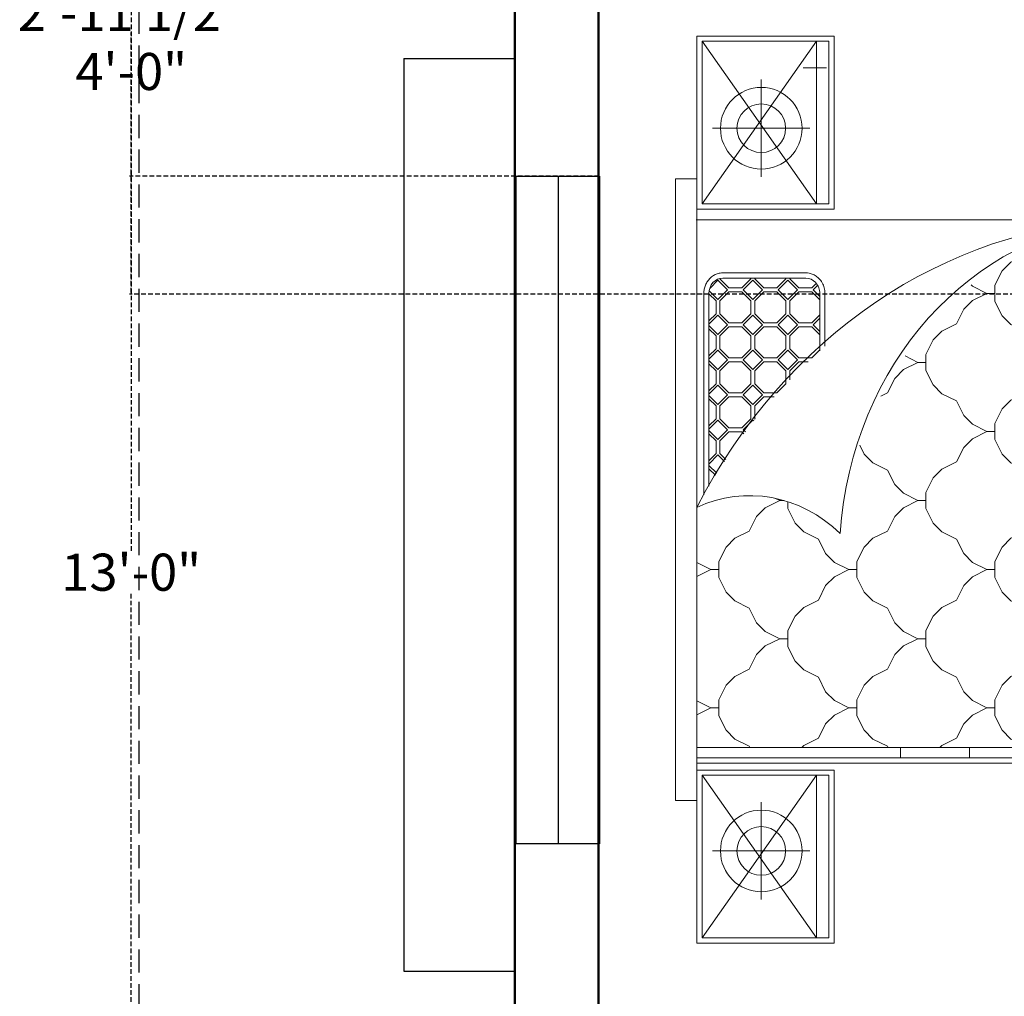
# Model space of a CAD drawing. Units: inches. Extents: x 513 to 1142, y 396 to 927.
# Tile 6 of 31: x 522 to 628, y 746 to 852. Entities that reach past the tile are written whole.
import ezdxf

# ---------------------------------------------------------------- set-up
doc = ezdxf.new("R2010")
doc.units = ezdxf.units.IN
doc.header["$MEASUREMENT"] = 0
doc.linetypes.add('DASHED', pattern=[0.75, 0.5, -0.25])
for name, color, linetype, lineweight in [('A-ANNO-DIMS', 2, 'DASHED', 18), ('A-WALL', 7, 'Continuous', 50), ('furniture', 92, 'Continuous', 18), ('windows', 172, 'Continuous', 25)]:
    doc.layers.add(name, color=color, linetype=linetype, lineweight=lineweight)
doc.styles.get("Standard").update_dxf_attribs({"font": 'arial.ttf'})
doc.dimstyles.get("Standard").update_dxf_attribs({"dimtxt": 4, "dimasz": 0.18, "dimexe": 0.18, "dimexo": 0.0625, "dimgap": 0.09, "dimtad": 0, "dimtih": 1, "dimtoh": 1, "dimdec": 0, "dimrnd": 6, "dimzin": 0, "dimdsep": 46, "dimlunit": 3, "dimtxsty": 'Standard', "dimcen": 0.09, "dimadec": 0, "dimazin": 0, "dimtfac": 1, "dimtdec": 0, "dimtofl": 0, "dimtmove": 0, "dimatfit": 3, "dimfxl": 1, "dimtolj": 1, "dimtzin": 0, "dimarcsym": 0})

# ---------------------------------------------------------------- blocks, each defined once
blk = doc.blocks.new('A$C029D5C69')
for p, q in [((0.4164, 2.0693), (0.4164, 2.0066)), ((2.2315, 2.0693), (0.4164, 2.0693)), ((2.2315, 2.0066), (2.2315, 2.0693)), ((0, 1.606), (0, 2.0066)), ((0, 2.0066), (0.505, 2.0066)), ((0.0151, 1.6211), (0.0151, 1.9915)), ((0.0151, 1.9915), (0.4899, 1.9915)), ((0.4164, 2.0066), (2.2315, 2.0066)), ((0.4899, 1.9915), (0.4899, 1.6211)), ((0.505, 2.0066), (0.505, 1.606)), ((0.5252, 0.0351), (0.5252, 2.0066)), ((0.5403, 0.0502), (0.5403, 2.0066)), ((0.5706, 0.0805), (0.5706, 2.0066)), ((0.6869, 1.966), (0.6666, 2.0066)), ((0.7072, 2.0066), (0.6869, 1.966)), ((1.0902, 1.966), (1.0699, 2.0066)), ((1.1106, 2.0066), (1.0902, 1.966)), ((1.8954, 1.9865), (1.3081, 1.9865)), ((2.1114, 2.0087), (2.1114, 0.0351)), ((2.6479, 2.0066), (2.1429, 2.0066)), ((2.1429, 2.0066), (2.1429, 1.606)), ((2.6328, 1.9915), (2.158, 1.9915)), ((2.158, 1.9915), (2.158, 1.6211)), ((2.6328, 1.6211), (2.6328, 1.9915)), ((2.6479, 1.606), (2.6479, 2.0066)), ((0.2689, 1.9609), (0.2689, 1.6764)), ((0.6869, 1.9425), (0.6869, 1.966)), ((0.6869, 1.9425), (0.6869, 1.966)), ((1.0902, 1.9425), (1.0902, 1.966)), ((1.0902, 1.9425), (1.0902, 1.966)), ((1.8954, 1.9713), (1.3339, 1.9713)), ((1.3849, 1.9713), (1.3656, 1.952)), ((1.3945, 1.9713), (1.3714, 1.9483)), ((1.4249, 1.945), (1.3986, 1.9713)), ((1.4288, 1.9507), (1.4081, 1.9713)), ((1.487, 1.9713), (1.4664, 1.9507)), ((1.4966, 1.9713), (1.4703, 1.945)), ((1.527, 1.945), (1.5007, 1.9713)), ((1.5309, 1.9507), (1.5102, 1.9713)), ((1.5891, 1.9713), (1.5685, 1.9507)), ((1.5987, 1.9713), (1.5724, 1.945)), ((1.6291, 1.945), (1.6028, 1.9713)), ((1.633, 1.9507), (1.6123, 1.9713)), ((1.6912, 1.9713), (1.6706, 1.9507)), ((1.7008, 1.9713), (1.6745, 1.945)), ((1.7312, 1.945), (1.7049, 1.9713)), ((1.7351, 1.9507), (1.7144, 1.9713)), ((1.7933, 1.9713), (1.7727, 1.9507)), ((1.8029, 1.9713), (1.7766, 1.945)), ((1.8333, 1.945), (1.807, 1.9713)), ((1.8372, 1.9507), (1.8165, 1.9713)), ((1.8954, 1.9713), (1.8748, 1.9507)), ((1.9043, 1.9707), (1.8787, 1.945)), ((1.9354, 1.945), (1.9114, 1.969)), ((2.379, 1.9609), (2.379, 1.6764)), ((0.6634, 1.9425), (0.621, 1.9213)), ((0.6634, 1.9425), (0.621, 1.9213)), ((0.6869, 1.9425), (0.6634, 1.9425)), ((0.6869, 1.9425), (0.7104, 1.9425)), ((0.7528, 1.9213), (0.7104, 1.9425)), ((0.7528, 1.9213), (0.7104, 1.9425)), ((1.0668, 1.9425), (1.0244, 1.9213)), ((1.0668, 1.9425), (1.0244, 1.9213)), ((1.0902, 1.9425), (1.0668, 1.9425)), ((1.0902, 1.9425), (1.1137, 1.9425)), ((1.1561, 1.9213), (1.1137, 1.9425)), ((1.1561, 1.9213), (1.1137, 1.9425)), ((1.4249, 1.945), (1.4059, 1.926)), ((1.4288, 1.9394), (1.4116, 1.9222)), ((1.4476, 1.9507), (1.4288, 1.9507)), ((1.4288, 1.9393), (1.4476, 1.9393)), ((1.4476, 1.9507), (1.4664, 1.9507)), ((1.4664, 1.9393), (1.4476, 1.9393)), ((1.493, 1.9128), (1.4664, 1.9394)), ((1.4986, 1.9167), (1.4703, 1.945)), ((1.527, 1.945), (1.4986, 1.9167)), ((1.5309, 1.9394), (1.5043, 1.9128)), ((1.5497, 1.9507), (1.5309, 1.9507)), ((1.5309, 1.9393), (1.5497, 1.9393)), ((1.5497, 1.9507), (1.5685, 1.9507)), ((1.5685, 1.9393), (1.5497, 1.9393)), ((1.595, 1.9128), (1.5685, 1.9394)), ((1.6007, 1.9167), (1.5724, 1.945)), ((1.6291, 1.945), (1.6007, 1.9167)), ((1.633, 1.9394), (1.6064, 1.9128)), ((1.6518, 1.9507), (1.633, 1.9507)), ((1.633, 1.9393), (1.6518, 1.9393)), ((1.6518, 1.9507), (1.6706, 1.9507)), ((1.6706, 1.9393), (1.6518, 1.9393)), ((1.6971, 1.9128), (1.6706, 1.9394)), ((1.7028, 1.9167), (1.6745, 1.945)), ((1.7312, 1.945), (1.7028, 1.9167)), ((1.7351, 1.9394), (1.7085, 1.9128)), ((1.7539, 1.9507), (1.7351, 1.9507)), ((1.7351, 1.9393), (1.7539, 1.9393)), ((1.7539, 1.9507), (1.7727, 1.9507)), ((1.7727, 1.9393), (1.7539, 1.9393)), ((1.7992, 1.9128), (1.7727, 1.9394)), ((1.8049, 1.9167), (1.7766, 1.945)), ((1.8333, 1.945), (1.8049, 1.9167)), ((1.8372, 1.9394), (1.8106, 1.9128)), ((1.856, 1.9507), (1.8372, 1.9507)), ((1.8372, 1.9393), (1.856, 1.9393)), ((1.856, 1.9507), (1.8748, 1.9507)), ((1.8748, 1.9393), (1.856, 1.9393)), ((1.9013, 1.9128), (1.8748, 1.9394)), ((1.907, 1.9167), (1.8787, 1.945)), ((1.9354, 1.945), (1.907, 1.9167)), ((1.9393, 1.9394), (1.9127, 1.9128)), ((1.9393, 1.9393), (1.9404, 1.9393)), ((1.9414, 1.688), (1.9414, 1.931)), ((1.9565, 1.688), (1.9565, 1.931)), ((0.621, 1.9213), (0.5955, 1.8958)), ((0.7783, 1.8958), (0.7528, 1.9213)), ((1.0243, 1.9213), (0.9988, 1.8958)), ((1.1816, 1.8958), (1.1561, 1.9213)), ((1.493, 1.8752), (1.493, 1.9128)), ((1.5043, 1.8752), (1.5043, 1.9128)), ((1.595, 1.8752), (1.595, 1.9128)), ((1.6064, 1.8752), (1.6064, 1.9128)), ((1.6971, 1.8752), (1.6971, 1.9128)), ((1.7085, 1.8752), (1.7085, 1.9128)), ((1.7992, 1.8752), (1.7992, 1.9128)), ((1.8106, 1.8752), (1.8106, 1.9128)), ((1.9013, 1.8752), (1.9013, 1.9128)), ((1.9127, 1.8752), (1.9127, 1.9128)), ((0.5955, 1.8958), (0.5743, 1.8534)), ((0.7995, 1.8534), (0.7783, 1.8958)), ((0.9989, 1.8958), (0.9777, 1.8534)), ((1.2028, 1.8534), (1.1816, 1.8958)), ((1.493, 1.8752), (1.4867, 1.869)), ((1.4986, 1.8713), (1.4922, 1.8648)), ((1.527, 1.8429), (1.4986, 1.8713)), ((1.5309, 1.8486), (1.5043, 1.8752)), ((1.595, 1.8752), (1.5685, 1.8486)), ((1.6007, 1.8713), (1.5724, 1.8429)), ((1.6291, 1.8429), (1.6007, 1.8713)), ((1.633, 1.8486), (1.6064, 1.8752)), ((1.6971, 1.8752), (1.6706, 1.8486)), ((1.7028, 1.8713), (1.6745, 1.8429)), ((1.7312, 1.8429), (1.7028, 1.8713)), ((1.7351, 1.8486), (1.7085, 1.8752)), ((1.7992, 1.8752), (1.7727, 1.8486)), ((1.8049, 1.8713), (1.7766, 1.8429)), ((1.8333, 1.8429), (1.8049, 1.8713)), ((1.8372, 1.8486), (1.8106, 1.8752)), ((1.9013, 1.8752), (1.8748, 1.8486)), ((1.907, 1.8713), (1.8787, 1.8429)), ((1.9354, 1.8429), (1.907, 1.8713)), ((1.9393, 1.8486), (1.9127, 1.8752)), ((0.5743, 1.8534), (0.5706, 1.8515)), ((0.5743, 1.8534), (0.5706, 1.8515)), ((0.8419, 1.8322), (0.7995, 1.8534)), ((0.8419, 1.8322), (0.7995, 1.8534)), ((0.9777, 1.8534), (0.9353, 1.8322)), ((0.9777, 1.8534), (0.9353, 1.8322)), ((1.2452, 1.8322), (1.2028, 1.8534)), ((1.2452, 1.8322), (1.2028, 1.8534)), ((1.527, 1.8429), (1.5242, 1.8401)), ((1.5497, 1.8486), (1.5309, 1.8486)), ((1.5497, 1.8486), (1.5685, 1.8486)), ((1.6007, 1.8146), (1.5724, 1.8429)), ((1.6291, 1.8429), (1.6007, 1.8146)), ((1.6518, 1.8486), (1.633, 1.8486)), ((1.6518, 1.8486), (1.6706, 1.8486)), ((1.7028, 1.8146), (1.6745, 1.8429)), ((1.7312, 1.8429), (1.7028, 1.8146)), ((1.7539, 1.8486), (1.7351, 1.8486)), ((1.7539, 1.8486), (1.7727, 1.8486)), ((1.8049, 1.8146), (1.7766, 1.8429)), ((1.8333, 1.8429), (1.8049, 1.8146)), ((1.856, 1.8486), (1.8372, 1.8486)), ((1.856, 1.8486), (1.8748, 1.8486)), ((1.907, 1.8146), (1.8787, 1.8429)), ((1.9354, 1.8429), (1.907, 1.8146)), ((1.9414, 1.8486), (1.9393, 1.8486)), ((0.1267, 1.8186), (0.4111, 1.8186)), ((0.8674, 1.8067), (0.8419, 1.8322)), ((0.9352, 1.8322), (0.9097, 1.8067)), ((1.2707, 1.8067), (1.2452, 1.8322)), ((1.5309, 1.8373), (1.5295, 1.8359)), ((1.5309, 1.8373), (1.5497, 1.8373)), ((1.5685, 1.8373), (1.5497, 1.8373)), ((1.595, 1.8107), (1.5685, 1.8373)), ((1.633, 1.8373), (1.6064, 1.8107)), ((1.633, 1.8373), (1.6518, 1.8373)), ((1.6706, 1.8373), (1.6518, 1.8373)), ((1.6971, 1.8107), (1.6706, 1.8373)), ((1.7351, 1.8373), (1.7085, 1.8107)), ((1.7351, 1.8373), (1.7539, 1.8373)), ((1.7727, 1.8373), (1.7539, 1.8373)), ((1.7992, 1.8107), (1.7727, 1.8373)), ((1.8372, 1.8373), (1.8106, 1.8107)), ((1.8372, 1.8373), (1.856, 1.8373)), ((1.8748, 1.8373), (1.856, 1.8373)), ((1.9013, 1.8107), (1.8748, 1.8373)), ((1.9393, 1.8373), (1.9127, 1.8107)), ((1.9393, 1.8373), (1.9414, 1.8373)), ((2.2367, 1.8186), (2.5212, 1.8186)), ((0.8886, 1.7643), (0.8674, 1.8067)), ((0.9098, 1.8067), (0.8886, 1.7643)), ((1.2919, 1.7643), (1.2707, 1.8067)), ((1.595, 1.7806), (1.595, 1.8107)), ((1.6064, 1.7731), (1.6064, 1.8107)), ((1.6971, 1.7731), (1.6971, 1.8107)), ((1.7085, 1.7731), (1.7085, 1.8107)), ((1.7992, 1.7731), (1.7992, 1.8107)), ((1.8106, 1.7731), (1.8106, 1.8107)), ((1.9013, 1.7731), (1.9013, 1.8107)), ((1.9127, 1.7731), (1.9127, 1.8107)), ((0.8886, 1.7408), (0.8886, 1.7643)), ((1.2981, 1.7768), (1.2919, 1.7643)), ((1.2919, 1.7519), (1.2919, 1.7643)), ((1.633, 1.7465), (1.6064, 1.7731)), ((1.6971, 1.7731), (1.6706, 1.7465)), ((1.7028, 1.7692), (1.6745, 1.7408)), ((1.7312, 1.7408), (1.7028, 1.7692)), ((1.7351, 1.7465), (1.7085, 1.7731)), ((1.7992, 1.7731), (1.7727, 1.7465)), ((1.8049, 1.7692), (1.7766, 1.7408)), ((1.8333, 1.7408), (1.8049, 1.7692)), ((1.8372, 1.7465), (1.8106, 1.7731)), ((1.9013, 1.7731), (1.8748, 1.7465)), ((1.907, 1.7692), (1.8787, 1.7408)), ((1.9354, 1.7408), (1.907, 1.7692)), ((1.9393, 1.7465), (1.9127, 1.7731)), ((0.8651, 1.7408), (0.8227, 1.7196)), ((0.8651, 1.7408), (0.8227, 1.7196)), ((0.912, 1.7408), (0.8651, 1.7408)), ((0.9544, 1.7196), (0.912, 1.7408)), ((0.9544, 1.7196), (0.912, 1.7408)), ((1.2684, 1.7408), (1.226, 1.7196)), ((1.2684, 1.7408), (1.226, 1.7196)), ((1.2885, 1.7408), (1.2684, 1.7408)), ((1.6518, 1.7465), (1.633, 1.7465)), ((1.6443, 1.7352), (1.6518, 1.7352)), ((1.6518, 1.7465), (1.6706, 1.7465)), ((1.6706, 1.7352), (1.6518, 1.7352)), ((1.6971, 1.7086), (1.6706, 1.7352)), ((1.7028, 1.7125), (1.6745, 1.7408)), ((1.7312, 1.7408), (1.7028, 1.7125)), ((1.7351, 1.7352), (1.7085, 1.7086)), ((1.7539, 1.7465), (1.7351, 1.7465)), ((1.7351, 1.7352), (1.7539, 1.7352)), ((1.7539, 1.7465), (1.7727, 1.7465)), ((1.7727, 1.7352), (1.7539, 1.7352)), ((1.7992, 1.7086), (1.7727, 1.7352)), ((1.8049, 1.7125), (1.7766, 1.7408)), ((1.8333, 1.7408), (1.8049, 1.7125)), ((1.8372, 1.7352), (1.8106, 1.7086)), ((1.856, 1.7465), (1.8372, 1.7465)), ((1.8372, 1.7352), (1.856, 1.7352)), ((1.856, 1.7465), (1.8748, 1.7465)), ((1.8748, 1.7352), (1.856, 1.7352)), ((1.9013, 1.7086), (1.8748, 1.7352)), ((1.907, 1.7125), (1.8787, 1.7408)), ((1.9354, 1.7408), (1.907, 1.7125)), ((1.9393, 1.7352), (1.9127, 1.7086)), ((1.9414, 1.7465), (1.9393, 1.7465)), ((1.9393, 1.7352), (1.9414, 1.7352)), ((0.5766, 1.6941), (0.5706, 1.7002)), ((0.8227, 1.7196), (0.7972, 1.6941)), ((0.98, 1.6941), (0.9545, 1.7196)), ((1.226, 1.7196), (1.2005, 1.6941)), ((1.6971, 1.682), (1.6971, 1.7086)), ((1.7085, 1.671), (1.7085, 1.7086)), ((1.7992, 1.671), (1.7992, 1.7086)), ((1.8106, 1.671), (1.8106, 1.7086)), ((1.9013, 1.671), (1.9013, 1.7086)), ((1.9127, 1.671), (1.9127, 1.7086)), ((0.5978, 1.6517), (0.5766, 1.6941)), ((0.7972, 1.6941), (0.776, 1.6517)), ((1.0011, 1.6517), (0.9799, 1.6941)), ((1.2005, 1.6941), (1.1793, 1.6517)), ((1.7318, 1.6477), (1.7085, 1.671)), ((1.7992, 1.671), (1.7759, 1.6477)), ((1.8339, 1.6477), (1.8106, 1.671)), ((1.9013, 1.671), (1.878, 1.6477)), ((1.926, 1.6577), (1.9127, 1.671)), ((2.5551, 1.6275), (2.5551, 1.696)), ((0.6402, 1.6305), (0.5978, 1.6517)), ((0.6402, 1.6305), (0.5978, 1.6517)), ((0.776, 1.6517), (0.7336, 1.6305)), ((0.776, 1.6517), (0.7336, 1.6305)), ((1.0435, 1.6305), (1.0011, 1.6517)), ((1.0435, 1.6305), (1.0011, 1.6517)), ((1.1793, 1.6517), (1.1369, 1.6305)), ((1.1793, 1.6517), (1.1369, 1.6305)), ((1.8961, 1.6477), (1.7289, 1.6477)), ((1.8049, 1.6671), (1.7855, 1.6477)), ((1.8244, 1.6477), (1.8049, 1.6671)), ((1.907, 1.6671), (1.8876, 1.6477)), ((1.9202, 1.6539), (1.907, 1.6671)), ((0.4899, 1.6211), (0.0151, 1.6211)), ((0.6657, 1.605), (0.6402, 1.6305)), ((0.7336, 1.6305), (0.7081, 1.605)), ((1.0691, 1.605), (1.0436, 1.6305)), ((1.1369, 1.6305), (1.1114, 1.605)), ((1.8961, 1.6325), (1.7422, 1.6325)), ((2.158, 1.6211), (2.6328, 1.6211)), ((0.505, 1.606), (0, 1.606)), ((0.6869, 1.5626), (0.6657, 1.605)), ((0.7081, 1.605), (0.6869, 1.5626)), ((1.0902, 1.5626), (1.069, 1.605)), ((1.1114, 1.605), (1.0902, 1.5626)), ((2.1429, 1.606), (2.6479, 1.606)), ((0.6869, 1.5392), (0.6869, 1.5626)), ((0.6869, 1.5392), (0.6869, 1.5626)), ((1.0902, 1.5392), (1.0902, 1.5626)), ((1.0902, 1.5392), (1.0902, 1.5626)), ((0.6634, 1.5391), (0.621, 1.5179)), ((0.6634, 1.5391), (0.621, 1.5179)), ((0.6869, 1.5392), (0.6634, 1.5392)), ((0.6869, 1.5392), (0.7104, 1.5392)), ((0.7528, 1.5179), (0.7104, 1.5391)), ((0.7528, 1.5179), (0.7104, 1.5391)), ((1.0668, 1.5391), (1.0244, 1.5179)), ((1.0668, 1.5391), (1.0244, 1.5179)), ((1.0902, 1.5392), (1.0668, 1.5392)), ((1.0902, 1.5392), (1.1137, 1.5392)), ((1.1561, 1.5179), (1.1137, 1.5391)), ((1.1561, 1.5179), (1.1137, 1.5391)), ((1.4534, 1.5308), (1.4277, 1.5179)), ((1.4534, 1.5308), (1.4277, 1.5179)), ((0.621, 1.5179), (0.5955, 1.4924)), ((0.7783, 1.4924), (0.7528, 1.5179)), ((1.0243, 1.5179), (0.9988, 1.4924)), ((1.1816, 1.4924), (1.1561, 1.5179)), ((1.4277, 1.5179), (1.4022, 1.4924)), ((0.5955, 1.4925), (0.5743, 1.4501)), ((0.7995, 1.4501), (0.7783, 1.4925)), ((0.9989, 1.4925), (0.9777, 1.4501)), ((1.2028, 1.4501), (1.1816, 1.4925)), ((1.4022, 1.4925), (1.381, 1.4501)), ((1.6062, 1.4501), (1.5966, 1.4692)), ((0.5743, 1.45), (0.5706, 1.4481)), ((0.5743, 1.45), (0.5706, 1.4481)), ((0.8419, 1.4288), (0.7995, 1.45)), ((0.8419, 1.4288), (0.7995, 1.45)), ((0.9777, 1.45), (0.9353, 1.4288)), ((0.9777, 1.45), (0.9353, 1.4288)), ((1.2452, 1.4288), (1.2028, 1.45)), ((1.2452, 1.4288), (1.2028, 1.45)), ((1.381, 1.45), (1.3386, 1.4288)), ((1.381, 1.45), (1.3386, 1.4288)), ((1.6486, 1.4288), (1.6062, 1.45)), ((1.6486, 1.4288), (1.6062, 1.45)), ((0.5403, 1.4117), (0.5706, 1.4117)), ((0.8674, 1.4033), (0.8419, 1.4288)), ((0.9352, 1.4288), (0.9097, 1.4033)), ((1.2707, 1.4033), (1.2452, 1.4288)), ((1.3386, 1.4288), (1.3131, 1.4033)), ((1.6741, 1.4033), (1.6486, 1.4288)), ((0.8886, 1.361), (0.8674, 1.4034)), ((0.9098, 1.4034), (0.8886, 1.361)), ((1.2919, 1.361), (1.2707, 1.4034)), ((1.3131, 1.4034), (1.2919, 1.361)), ((1.6953, 1.361), (1.6741, 1.4034)), ((1.714, 1.3984), (1.6953, 1.361)), ((0.8886, 1.3375), (0.8886, 1.3609)), ((1.2919, 1.3375), (1.2919, 1.3609)), ((1.6953, 1.3375), (1.6953, 1.3609)), ((0.8651, 1.3374), (0.8227, 1.3162)), ((0.8651, 1.3374), (0.8227, 1.3162)), ((0.912, 1.3375), (0.8651, 1.3375)), ((0.9544, 1.3162), (0.912, 1.3374)), ((0.9544, 1.3162), (0.912, 1.3374)), ((1.2684, 1.3374), (1.226, 1.3162)), ((1.2684, 1.3374), (1.226, 1.3162)), ((1.3154, 1.3375), (1.2684, 1.3375)), ((1.3578, 1.3162), (1.3154, 1.3374)), ((1.3578, 1.3162), (1.3154, 1.3374)), ((1.6718, 1.3374), (1.6294, 1.3162)), ((1.6718, 1.3374), (1.6294, 1.3162)), ((1.7187, 1.3375), (1.6718, 1.3375)), ((1.7611, 1.3162), (1.7187, 1.3374)), ((1.7611, 1.3162), (1.7187, 1.3374)), ((0.5766, 1.2908), (0.5706, 1.2968)), ((0.8227, 1.3163), (0.7972, 1.2908)), ((0.98, 1.2908), (0.9545, 1.3163)), ((1.226, 1.3163), (1.2005, 1.2908)), ((1.3833, 1.2908), (1.3578, 1.3163)), ((1.6294, 1.3163), (1.6039, 1.2908)), ((1.7867, 1.2908), (1.7611, 1.3163)), ((0.5978, 1.2484), (0.5766, 1.2908)), ((0.7972, 1.2908), (0.776, 1.2484)), ((1.0011, 1.2484), (0.9799, 1.2908)), ((1.2005, 1.2908), (1.1793, 1.2484)), ((1.4045, 1.2484), (1.3833, 1.2908)), ((1.6039, 1.2908), (1.5827, 1.2484)), ((1.8078, 1.2484), (1.7866, 1.2908)), ((0.6402, 1.2271), (0.5978, 1.2483)), ((0.6402, 1.2271), (0.5978, 1.2483)), ((0.776, 1.2483), (0.7336, 1.2271)), ((0.776, 1.2483), (0.7336, 1.2271)), ((1.0435, 1.2271), (1.0011, 1.2483)), ((1.0435, 1.2271), (1.0011, 1.2483)), ((1.1793, 1.2483), (1.1369, 1.2271)), ((1.1793, 1.2483), (1.1369, 1.2271)), ((1.4469, 1.2271), (1.4045, 1.2483)), ((1.4469, 1.2271), (1.4045, 1.2483)), ((1.5827, 1.2483), (1.5403, 1.2271)), ((1.5827, 1.2483), (1.5403, 1.2271)), ((1.8502, 1.2271), (1.8078, 1.2483)), ((1.8502, 1.2271), (1.8078, 1.2483)), ((0.5403, 1.21), (0.5706, 1.21)), ((0.6657, 1.2017), (0.6402, 1.2272)), ((0.7336, 1.2272), (0.7081, 1.2017)), ((1.0691, 1.2017), (1.0436, 1.2272)), ((1.1369, 1.2272), (1.1114, 1.2017)), ((1.4724, 1.2017), (1.4469, 1.2272)), ((1.5403, 1.2272), (1.5148, 1.2017)), ((1.8758, 1.2017), (1.8503, 1.2272)), ((0.6869, 1.1593), (0.6657, 1.2017)), ((0.7081, 1.2017), (0.6869, 1.1593)), ((1.0902, 1.1593), (1.069, 1.2017)), ((1.1114, 1.2017), (1.0902, 1.1593)), ((1.4936, 1.1593), (1.4724, 1.2017)), ((1.5148, 1.2017), (1.4936, 1.1593)), ((1.8969, 1.1593), (1.8757, 1.2017)), ((1.9181, 1.2017), (1.8969, 1.1593)), ((1.9215, 1.2051), (1.9181, 1.2017)), ((0.6869, 1.1358), (0.6869, 1.1593)), ((0.6869, 1.1358), (0.6869, 1.1593)), ((1.0902, 1.1358), (1.0902, 1.1593)), ((1.0902, 1.1358), (1.0902, 1.1593)), ((1.4936, 1.1358), (1.4936, 1.1593)), ((1.4936, 1.1358), (1.4936, 1.1593)), ((1.8969, 1.1358), (1.8969, 1.1593)), ((1.8969, 1.1358), (1.8969, 1.1593)), ((0.6634, 1.1358), (0.621, 1.1146)), ((0.6634, 1.1358), (0.621, 1.1146)), ((0.6869, 1.1358), (0.6634, 1.1358)), ((0.6869, 1.1358), (0.7104, 1.1358)), ((0.7528, 1.1146), (0.7104, 1.1358)), ((0.7528, 1.1146), (0.7104, 1.1358)), ((1.0668, 1.1358), (1.0244, 1.1146)), ((1.0668, 1.1358), (1.0244, 1.1146)), ((1.0902, 1.1358), (1.0668, 1.1358)), ((1.0902, 1.1358), (1.1137, 1.1358)), ((1.1561, 1.1146), (1.1137, 1.1358)), ((1.1561, 1.1146), (1.1137, 1.1358)), ((1.4701, 1.1358), (1.4277, 1.1146)), ((1.4701, 1.1358), (1.4277, 1.1146)), ((1.4936, 1.1358), (1.4701, 1.1358)), ((1.4936, 1.1358), (1.5171, 1.1358)), ((1.5595, 1.1146), (1.5171, 1.1358)), ((1.5595, 1.1146), (1.5171, 1.1358)), ((1.8735, 1.1358), (1.8311, 1.1146)), ((1.8735, 1.1358), (1.8311, 1.1146)), ((1.8969, 1.1358), (1.8735, 1.1358)), ((1.8969, 1.1358), (1.9204, 1.1358)), ((1.9628, 1.1146), (1.9204, 1.1358)), ((1.9628, 1.1146), (1.9204, 1.1358)), ((0.621, 1.1146), (0.5955, 1.0891)), ((0.7783, 1.0891), (0.7528, 1.1146)), ((1.0243, 1.1146), (0.9988, 1.0891)), ((1.1816, 1.0891), (1.1561, 1.1146)), ((1.4277, 1.1146), (1.4022, 1.0891)), ((1.585, 1.0891), (1.5595, 1.1146)), ((1.831, 1.1146), (1.8055, 1.0891)), ((1.9883, 1.0891), (1.9628, 1.1146)), ((0.5955, 1.0891), (0.5743, 1.0467)), ((0.7995, 1.0467), (0.7783, 1.0891)), ((0.9989, 1.0891), (0.9777, 1.0467)), ((1.2028, 1.0467), (1.1816, 1.0891)), ((1.4022, 1.0891), (1.381, 1.0467)), ((1.6062, 1.0467), (1.585, 1.0891)), ((1.8056, 1.0891), (1.7844, 1.0467)), ((2.0095, 1.0467), (1.9883, 1.0891)), ((0.5743, 1.0467), (0.5706, 1.0448)), ((0.5743, 1.0467), (0.5706, 1.0448)), ((0.8419, 1.0255), (0.7995, 1.0467)), ((0.8419, 1.0255), (0.7995, 1.0467)), ((0.9777, 1.0467), (0.9353, 1.0255)), ((0.9777, 1.0467), (0.9353, 1.0255)), ((1.2452, 1.0255), (1.2028, 1.0467)), ((1.2452, 1.0255), (1.2028, 1.0467)), ((1.381, 1.0467), (1.3386, 1.0255)), ((1.381, 1.0467), (1.3386, 1.0255)), ((1.6486, 1.0255), (1.6062, 1.0467)), ((1.6486, 1.0255), (1.6062, 1.0467)), ((1.7844, 1.0467), (1.742, 1.0255)), ((1.7844, 1.0467), (1.742, 1.0255)), ((2.0276, 1.0376), (2.0095, 1.0467)), ((2.0276, 1.0376), (2.0095, 1.0467)), ((0.8674, 1), (0.8419, 1.0255)), ((0.9352, 1.0255), (0.9097, 1)), ((1.2707, 1), (1.2452, 1.0255)), ((1.3386, 1.0255), (1.3131, 1)), ((1.6741, 1), (1.6486, 1.0255)), ((1.7419, 1.0255), (1.7164, 1)), ((0.8886, 0.9576), (0.8674, 1)), ((0.9098, 1), (0.8886, 0.9576)), ((1.2919, 0.9576), (1.2707, 1)), ((1.3131, 1), (1.2919, 0.9576)), ((1.6953, 0.9576), (1.6741, 1)), ((1.7165, 1), (1.6953, 0.9576)), ((0.8886, 0.9341), (0.8886, 0.9576)), ((1.2919, 0.9341), (1.2919, 0.9576)), ((1.6953, 0.9341), (1.6953, 0.9576)), ((0.8651, 0.9341), (0.8227, 0.9129)), ((0.8651, 0.9341), (0.8227, 0.9129)), ((0.912, 0.9341), (0.8651, 0.9341)), ((0.9544, 0.9129), (0.912, 0.9341)), ((0.9544, 0.9129), (0.912, 0.9341)), ((1.2684, 0.9341), (1.226, 0.9129)), ((1.2684, 0.9341), (1.226, 0.9129)), ((1.3154, 0.9341), (1.2684, 0.9341)), ((1.3578, 0.9129), (1.3154, 0.9341)), ((1.3578, 0.9129), (1.3154, 0.9341)), ((1.6718, 0.9341), (1.6294, 0.9129)), ((1.6718, 0.9341), (1.6294, 0.9129)), ((1.7187, 0.9341), (1.6718, 0.9341)), ((1.7611, 0.9129), (1.7187, 0.9341)), ((1.7611, 0.9129), (1.7187, 0.9341)), ((2.066, 0.9295), (2.0327, 0.9129)), ((2.066, 0.9295), (2.0327, 0.9129)), ((2.066, 0.9457), (2.066, 0.0805)), ((0.5766, 0.8874), (0.5706, 0.8935)), ((0.8227, 0.9129), (0.7972, 0.8874)), ((0.98, 0.8874), (0.9545, 0.9129)), ((1.226, 0.9129), (1.2005, 0.8874)), ((1.3833, 0.8874), (1.3578, 0.9129)), ((1.6294, 0.9129), (1.6039, 0.8874)), ((1.7867, 0.8874), (1.7611, 0.9129)), ((2.0327, 0.9129), (2.0072, 0.8874)), ((0.5978, 0.845), (0.5766, 0.8874)), ((0.7972, 0.8874), (0.776, 0.845)), ((1.0011, 0.845), (0.9799, 0.8874)), ((1.2005, 0.8874), (1.1793, 0.845)), ((1.4045, 0.845), (1.3833, 0.8874)), ((1.6039, 0.8874), (1.5827, 0.845)), ((1.8078, 0.845), (1.7866, 0.8874)), ((2.0072, 0.8874), (1.986, 0.845)), ((0.6402, 0.8238), (0.5978, 0.845)), ((0.6402, 0.8238), (0.5978, 0.845)), ((0.776, 0.845), (0.7336, 0.8238)), ((0.776, 0.845), (0.7336, 0.8238)), ((1.0435, 0.8238), (1.0011, 0.845)), ((1.0435, 0.8238), (1.0011, 0.845)), ((1.1793, 0.845), (1.1369, 0.8238)), ((1.1793, 0.845), (1.1369, 0.8238)), ((1.4469, 0.8238), (1.4045, 0.845)), ((1.4469, 0.8238), (1.4045, 0.845)), ((1.5827, 0.845), (1.5403, 0.8238)), ((1.5827, 0.845), (1.5403, 0.8238)), ((1.8502, 0.8238), (1.8078, 0.845)), ((1.8502, 0.8238), (1.8078, 0.845)), ((1.986, 0.845), (1.9436, 0.8238)), ((1.986, 0.845), (1.9436, 0.8238)), ((2.0962, 0.8369), (2.0962, 0.0502)), ((0.6657, 0.7983), (0.6402, 0.8238)), ((0.7336, 0.8238), (0.7081, 0.7983)), ((1.0691, 0.7983), (1.0436, 0.8238)), ((1.1369, 0.8238), (1.1114, 0.7983)), ((1.4724, 0.7983), (1.4469, 0.8238)), ((1.5403, 0.8238), (1.5148, 0.7983)), ((1.8758, 0.7983), (1.8503, 0.8238)), ((1.9436, 0.8238), (1.9181, 0.7983)), ((0.6869, 0.7559), (0.6657, 0.7983)), ((0.7081, 0.7983), (0.6869, 0.7559)), ((1.0902, 0.7559), (1.069, 0.7983)), ((1.1114, 0.7983), (1.0902, 0.7559)), ((1.4936, 0.7559), (1.4724, 0.7983)), ((1.5148, 0.7983), (1.4936, 0.7559)), ((1.8969, 0.7559), (1.8757, 0.7983)), ((1.9181, 0.7983), (1.8969, 0.7559)), ((0.6869, 0.7325), (0.6869, 0.7559)), ((0.6869, 0.7325), (0.6869, 0.7559)), ((1.0902, 0.7325), (1.0902, 0.7559)), ((1.0902, 0.7325), (1.0902, 0.7559)), ((1.2024, 0.7028), (1.2503, 0.7507)), ((1.4936, 0.7325), (1.4936, 0.7559)), ((1.4936, 0.7325), (1.4936, 0.7559)), ((1.8969, 0.7325), (1.8969, 0.7559)), ((1.8969, 0.7325), (1.8969, 0.7559)), ((0.6634, 0.7324), (0.621, 0.7112)), ((0.6634, 0.7324), (0.621, 0.7112)), ((0.6869, 0.7325), (0.6634, 0.7325)), ((0.6869, 0.7325), (0.7104, 0.7325)), ((0.7528, 0.7112), (0.7104, 0.7324)), ((0.7528, 0.7112), (0.7104, 0.7324)), ((1.0668, 0.7324), (1.0244, 0.7112)), ((1.0668, 0.7324), (1.0244, 0.7112)), ((1.0902, 0.7325), (1.0668, 0.7325)), ((1.0902, 0.7325), (1.1137, 0.7325)), ((1.1561, 0.7112), (1.1137, 0.7324)), ((1.1561, 0.7112), (1.1137, 0.7324)), ((1.4701, 0.7324), (1.4277, 0.7112)), ((1.4701, 0.7324), (1.4277, 0.7112)), ((1.4936, 0.7325), (1.4701, 0.7325)), ((1.4936, 0.7325), (1.5171, 0.7325)), ((1.5595, 0.7112), (1.5171, 0.7324)), ((1.5595, 0.7112), (1.5171, 0.7324)), ((1.8735, 0.7324), (1.8311, 0.7112)), ((1.8735, 0.7324), (1.8311, 0.7112)), ((1.8969, 0.7325), (1.8735, 0.7325)), ((1.8969, 0.7325), (1.9204, 0.7325)), ((1.9628, 0.7112), (1.9204, 0.7324)), ((1.9628, 0.7112), (1.9204, 0.7324)), ((0.621, 0.7113), (0.5955, 0.6858)), ((0.7783, 0.6858), (0.7528, 0.7113)), ((1.0243, 0.7113), (0.9988, 0.6858)), ((1.1816, 0.6858), (1.1561, 0.7113)), ((1.4277, 0.7113), (1.4022, 0.6858)), ((1.585, 0.6858), (1.5595, 0.7113)), ((1.831, 0.7113), (1.8055, 0.6858)), ((1.9883, 0.6858), (1.9628, 0.7113)), ((0.5955, 0.6858), (0.5743, 0.6434)), ((0.7995, 0.6434), (0.7783, 0.6858)), ((0.9989, 0.6858), (0.9777, 0.6434)), ((1.2028, 0.6434), (1.1816, 0.6858)), ((1.4022, 0.6858), (1.381, 0.6434)), ((1.6062, 0.6434), (1.585, 0.6858)), ((1.8056, 0.6858), (1.7844, 0.6434)), ((2.0095, 0.6434), (1.9883, 0.6858)), ((0.5743, 0.6433), (0.5706, 0.6414)), ((0.5743, 0.6433), (0.5706, 0.6414)), ((0.8419, 0.6221), (0.7995, 0.6433)), ((0.8419, 0.6221), (0.7995, 0.6433)), ((0.9777, 0.6433), (0.9353, 0.6221)), ((0.9777, 0.6433), (0.9353, 0.6221)), ((1.2452, 0.6221), (1.2028, 0.6433)), ((1.2452, 0.6221), (1.2028, 0.6433)), ((1.381, 0.6433), (1.3386, 0.6221)), ((1.381, 0.6433), (1.3386, 0.6221)), ((1.6486, 0.6221), (1.6062, 0.6433)), ((1.6486, 0.6221), (1.6062, 0.6433)), ((1.7844, 0.6433), (1.742, 0.6221)), ((1.7844, 0.6433), (1.742, 0.6221)), ((2.0519, 0.6221), (2.0095, 0.6433)), ((2.0519, 0.6221), (2.0095, 0.6433)), ((0.8674, 0.5967), (0.8419, 0.6222)), ((0.9352, 0.6222), (0.9097, 0.5967)), ((1.2707, 0.5967), (1.2452, 0.6222)), ((1.3386, 0.6222), (1.3131, 0.5967)), ((1.6741, 0.5967), (1.6486, 0.6222)), ((1.7419, 0.6222), (1.7164, 0.5967)), ((2.066, 0.6081), (2.0519, 0.6222)), ((0.8886, 0.5543), (0.8674, 0.5967)), ((0.9098, 0.5967), (0.8886, 0.5543)), ((1.2919, 0.5543), (1.2707, 0.5967)), ((1.3131, 0.5967), (1.2919, 0.5543)), ((1.6953, 0.5543), (1.6741, 0.5967)), ((1.7165, 0.5967), (1.6953, 0.5543)), ((0.8886, 0.5308), (0.8886, 0.5543)), ((1.2919, 0.5308), (1.2919, 0.5543)), ((1.6953, 0.5308), (1.6953, 0.5543)), ((0.8651, 0.5308), (0.8227, 0.5096)), ((0.8651, 0.5308), (0.8227, 0.5096)), ((0.912, 0.5308), (0.8651, 0.5308)), ((0.9544, 0.5096), (0.912, 0.5308)), ((0.9544, 0.5096), (0.912, 0.5308)), ((1.2684, 0.5308), (1.226, 0.5096)), ((1.2684, 0.5308), (1.226, 0.5096)), ((1.3154, 0.5308), (1.2684, 0.5308)), ((1.3578, 0.5096), (1.3154, 0.5308)), ((1.3578, 0.5096), (1.3154, 0.5308)), ((1.6718, 0.5308), (1.6294, 0.5096)), ((1.6718, 0.5308), (1.6294, 0.5096)), ((1.7187, 0.5308), (1.6718, 0.5308)), ((1.7611, 0.5096), (1.7187, 0.5308)), ((1.7611, 0.5096), (1.7187, 0.5308)), ((2.066, 0.5262), (2.0327, 0.5096)), ((2.066, 0.5262), (2.0327, 0.5096)), ((0.5766, 0.4841), (0.5706, 0.4901)), ((0.8227, 0.5096), (0.7972, 0.4841)), ((0.98, 0.4841), (0.9545, 0.5096)), ((1.226, 0.5096), (1.2005, 0.4841)), ((1.3833, 0.4841), (1.3578, 0.5096)), ((1.6294, 0.5096), (1.6039, 0.4841)), ((1.7867, 0.4841), (1.7611, 0.5096)), ((2.0327, 0.5096), (2.0072, 0.4841)), ((0.5978, 0.4417), (0.5766, 0.4841)), ((0.7972, 0.4841), (0.776, 0.4417)), ((1.0011, 0.4417), (0.9799, 0.4841)), ((1.2005, 0.4841), (1.1793, 0.4417)), ((1.4045, 0.4417), (1.3833, 0.4841)), ((1.6039, 0.4841), (1.5827, 0.4417)), ((1.8078, 0.4417), (1.7866, 0.4841)), ((2.0072, 0.4841), (1.986, 0.4417)), ((0.6402, 0.4205), (0.5978, 0.4417)), ((0.6402, 0.4205), (0.5978, 0.4417)), ((0.776, 0.4417), (0.7336, 0.4205)), ((0.776, 0.4417), (0.7336, 0.4205)), ((1.0435, 0.4205), (1.0011, 0.4417)), ((1.0435, 0.4205), (1.0011, 0.4417)), ((1.1793, 0.4417), (1.1369, 0.4205)), ((1.1793, 0.4417), (1.1369, 0.4205)), ((1.4469, 0.4205), (1.4045, 0.4417)), ((1.4469, 0.4205), (1.4045, 0.4417)), ((1.5827, 0.4417), (1.5403, 0.4205)), ((1.5827, 0.4417), (1.5403, 0.4205)), ((1.8502, 0.4205), (1.8078, 0.4417)), ((1.8502, 0.4205), (1.8078, 0.4417)), ((1.986, 0.4417), (1.9436, 0.4205)), ((1.986, 0.4417), (1.9436, 0.4205)), ((0.6657, 0.395), (0.6402, 0.4205)), ((0.7336, 0.4205), (0.7081, 0.395)), ((1.0691, 0.395), (1.0436, 0.4205)), ((1.1369, 0.4205), (1.1114, 0.395)), ((1.4724, 0.395), (1.4469, 0.4205)), ((1.5403, 0.4205), (1.5148, 0.395)), ((1.8758, 0.395), (1.8503, 0.4205)), ((1.9436, 0.4205), (1.9181, 0.395)), ((0.6869, 0.3526), (0.6657, 0.395)), ((0.7081, 0.395), (0.6869, 0.3526)), ((1.0902, 0.3526), (1.069, 0.395)), ((1.1114, 0.395), (1.0902, 0.3526)), ((1.4936, 0.3526), (1.4724, 0.395)), ((1.5148, 0.395), (1.4936, 0.3526)), ((1.8969, 0.3526), (1.8757, 0.395)), ((1.9181, 0.395), (1.8969, 0.3526)), ((0.6869, 0.3291), (0.6869, 0.3526)), ((0.6869, 0.3291), (0.6869, 0.3526)), ((1.0902, 0.3291), (1.0902, 0.3526)), ((1.0902, 0.3291), (1.0902, 0.3526)), ((1.4936, 0.3291), (1.4936, 0.3526)), ((1.4936, 0.3291), (1.4936, 0.3526)), ((1.8969, 0.3291), (1.8969, 0.3526)), ((1.8969, 0.3291), (1.8969, 0.3526)), ((0.6634, 0.3291), (0.621, 0.3079)), ((0.6634, 0.3291), (0.621, 0.3079)), ((0.6869, 0.3291), (0.6634, 0.3291)), ((0.6869, 0.3291), (0.7104, 0.3291)), ((0.7528, 0.3079), (0.7104, 0.3291)), ((0.7528, 0.3079), (0.7104, 0.3291)), ((1.0668, 0.3291), (1.0244, 0.3079)), ((1.0668, 0.3291), (1.0244, 0.3079)), ((1.0902, 0.3291), (1.0668, 0.3291)), ((1.0902, 0.3291), (1.1137, 0.3291)), ((1.1561, 0.3079), (1.1137, 0.3291)), ((1.1561, 0.3079), (1.1137, 0.3291)), ((1.4701, 0.3291), (1.4277, 0.3079)), ((1.4701, 0.3291), (1.4277, 0.3079)), ((1.4936, 0.3291), (1.4701, 0.3291)), ((1.4936, 0.3291), (1.5171, 0.3291)), ((1.5595, 0.3079), (1.5171, 0.3291)), ((1.5595, 0.3079), (1.5171, 0.3291)), ((1.8735, 0.3291), (1.8311, 0.3079)), ((1.8735, 0.3291), (1.8311, 0.3079)), ((1.8969, 0.3291), (1.8735, 0.3291)), ((1.8969, 0.3291), (1.9204, 0.3291)), ((1.9628, 0.3079), (1.9204, 0.3291)), ((1.9628, 0.3079), (1.9204, 0.3291)), ((0.621, 0.3079), (0.5955, 0.2824)), ((0.7783, 0.2824), (0.7528, 0.3079)), ((1.0243, 0.3079), (0.9988, 0.2824)), ((1.1816, 0.2824), (1.1561, 0.3079)), ((1.4277, 0.3079), (1.4022, 0.2824)), ((1.585, 0.2824), (1.5595, 0.3079)), ((1.831, 0.3079), (1.8055, 0.2824)), ((1.9883, 0.2824), (1.9628, 0.3079)), ((0.5955, 0.2824), (0.5743, 0.24)), ((0.7995, 0.24), (0.7783, 0.2824)), ((0.9989, 0.2824), (0.9777, 0.24)), ((1.2028, 0.24), (1.1816, 0.2824)), ((1.4022, 0.2824), (1.381, 0.24)), ((1.6062, 0.24), (1.585, 0.2824)), ((1.8056, 0.2824), (1.7844, 0.24)), ((2.0095, 0.24), (1.9883, 0.2824)), ((0.5743, 0.24), (0.5706, 0.2381)), ((0.5743, 0.24), (0.5706, 0.2381)), ((0.8419, 0.2188), (0.7995, 0.24)), ((0.8419, 0.2188), (0.7995, 0.24)), ((0.9777, 0.24), (0.9353, 0.2188)), ((0.9777, 0.24), (0.9353, 0.2188)), ((1.2452, 0.2188), (1.2028, 0.24)), ((1.2452, 0.2188), (1.2028, 0.24)), ((1.381, 0.24), (1.3386, 0.2188)), ((1.381, 0.24), (1.3386, 0.2188)), ((1.6486, 0.2188), (1.6062, 0.24)), ((1.6486, 0.2188), (1.6062, 0.24)), ((1.7844, 0.24), (1.742, 0.2188)), ((1.7844, 0.24), (1.742, 0.2188)), ((2.0519, 0.2188), (2.0095, 0.24)), ((2.0519, 0.2188), (2.0095, 0.24)), ((0.8674, 0.1933), (0.8419, 0.2188)), ((0.9352, 0.2188), (0.9097, 0.1933)), ((1.2707, 0.1933), (1.2452, 0.2188)), ((1.3386, 0.2188), (1.3131, 0.1933)), ((1.6741, 0.1933), (1.6486, 0.2188)), ((1.7419, 0.2188), (1.7164, 0.1933)), ((2.066, 0.2047), (2.0519, 0.2188)), ((0.8886, 0.1509), (0.8674, 0.1933)), ((0.9098, 0.1933), (0.8886, 0.1509)), ((1.2919, 0.1509), (1.2707, 0.1933)), ((1.3131, 0.1933), (1.2919, 0.1509)), ((1.6953, 0.1509), (1.6741, 0.1933)), ((1.7165, 0.1933), (1.6953, 0.1509)), ((0.8886, 0.1275), (0.8886, 0.1509)), ((1.2919, 0.1275), (1.2919, 0.1509)), ((1.6953, 0.1275), (1.6953, 0.1509)), ((0.8651, 0.1274), (0.8227, 0.1062)), ((0.8651, 0.1274), (0.8227, 0.1062)), ((0.912, 0.1275), (0.8651, 0.1275)), ((0.9544, 0.1062), (0.912, 0.1274)), ((0.9544, 0.1062), (0.912, 0.1274)), ((1.2684, 0.1274), (1.226, 0.1062)), ((1.2684, 0.1274), (1.226, 0.1062)), ((1.3154, 0.1275), (1.2684, 0.1275)), ((1.3578, 0.1062), (1.3154, 0.1274)), ((1.3578, 0.1062), (1.3154, 0.1274)), ((1.6718, 0.1274), (1.6294, 0.1062)), ((1.6718, 0.1274), (1.6294, 0.1062)), ((1.7187, 0.1275), (1.6718, 0.1275)), ((1.7611, 0.1062), (1.7187, 0.1274)), ((1.7611, 0.1062), (1.7187, 0.1274)), ((2.066, 0.1228), (2.0327, 0.1062)), ((2.066, 0.1228), (2.0327, 0.1062)), ((0.5766, 0.0807), (0.5706, 0.0868)), ((0.8227, 0.1062), (0.7972, 0.0807)), ((0.98, 0.0807), (0.9545, 0.1062)), ((1.226, 0.1062), (1.2005, 0.0807)), ((1.3833, 0.0807), (1.3578, 0.1062)), ((1.6294, 0.1062), (1.6039, 0.0807)), ((1.7867, 0.0807), (1.7611, 0.1062)), ((2.0327, 0.1062), (2.0072, 0.0807)), ((0.5978, 0.0384), (0.5766, 0.0808)), ((0.7972, 0.0808), (0.776, 0.0384)), ((1.0011, 0.0384), (0.9799, 0.0808)), ((1.2005, 0.0808), (1.1793, 0.0384)), ((1.4045, 0.0384), (1.3833, 0.0808)), ((1.6039, 0.0808), (1.5827, 0.0384)), ((1.8078, 0.0384), (1.7866, 0.0808)), ((2.0072, 0.0808), (1.986, 0.0384)), ((0.6402, 0.0171), (0.5978, 0.0383)), ((0.6402, 0.0171), (0.5978, 0.0383)), ((2.0309, 0.0454), (0.6056, 0.0454)), ((0.776, 0.0383), (0.7336, 0.0171)), ((0.776, 0.0383), (0.7336, 0.0171)), ((1.0435, 0.0171), (1.0011, 0.0383)), ((1.0435, 0.0171), (1.0011, 0.0383)), ((1.1793, 0.0383), (1.1369, 0.0171)), ((1.1793, 0.0383), (1.1369, 0.0171)), ((1.4469, 0.0171), (1.4045, 0.0383)), ((1.4469, 0.0171), (1.4045, 0.0383)), ((1.5827, 0.0383), (1.5403, 0.0171)), ((1.5827, 0.0383), (1.5403, 0.0171)), ((1.8502, 0.0171), (1.8078, 0.0383)), ((1.8502, 0.0171), (1.8078, 0.0383)), ((1.986, 0.0383), (1.9436, 0.0171)), ((1.986, 0.0383), (1.9436, 0.0171)), ((2.0763, 0), (0.5603, 0)), ((2.0612, 0.0151), (0.5754, 0.0151)), ((0.6523, 0.005), (0.6402, 0.0171)), ((0.7336, 0.0171), (0.7215, 0.005)), ((1.0557, 0.005), (1.0436, 0.0171)), ((1.1369, 0.0171), (1.1248, 0.005)), ((1.459, 0.005), (1.4469, 0.0171)), ((1.5403, 0.0171), (1.5282, 0.005)), ((1.8623, 0.005), (1.8503, 0.0171)), ((1.9436, 0.0171), (1.9315, 0.005))]:
    blk.add_line(p, q)
at = {"ltscale": 0.005}
for p, q in [((0.4899, 1.6568), (0.0151, 1.9915)), ((0.0151, 1.6568), (0.4899, 1.9915)), ((2.6328, 1.6568), (2.158, 1.9915)), ((2.158, 1.6568), (2.6328, 1.9915)), ((0.0151, 1.6568), (0.4899, 1.6568)), ((2.6328, 1.6568), (2.158, 1.6568))]:
    blk.add_line(p, q, dxfattribs=at)
for centre, radius in [((0.2689, 1.8186), 0.1191), ((2.379, 1.8186), 0.1191), ((0.2689, 1.8186), 0.0711), ((2.379, 1.8186), 0.0711)]:
    blk.add_circle(centre, radius)
for centre, radius, start, end in [((0.2843, 0.0157), 0.6251, 10.2961, 13.2684), ((0.6056, 0.0805), 0.0351, 180, 270), ((2.0309, 0.0805), 0.0351, 270, 0), ((0.5603, 0.0351), 0.0351, 180, 270), ((0.5754, 0.0502), 0.0351, 180, 270), ((2.0612, 0.0502), 0.0351, 270, 0), ((2.0763, 0.0351), 0.0351, 270, 0)]:
    blk.add_arc(centre, radius, start, end)
for centre, major_axis, ratio, start_param, end_param in [((0.8506, 1.8527), (-0.4556, 0), 0.89, 2.430919, 3.53111), ((0.3667, 0.6698), (1.7398, 0.1668), 0.88072, -0.045073, 0.941433), ((1.8961, 1.931), (-0.0453, 0), 0.89, 3.141593, 4.712389), ((1.8961, 1.688), (-0.0453, 0), 0.89, 1.570796, 3.141593), ((1.0874, 0.6748), (1.021, 0.1213), 0.889348, -0.031673, 1.359628)]:
    blk.add_ellipse(centre, major_axis=major_axis, ratio=ratio, start_param=start_param, end_param=end_param)
for points, knots in [([(1.9565, 1.931), (1.9565, 1.9336), (1.9563, 1.9362), (1.9553, 1.9428), (1.9543, 1.9467), (1.9512, 1.9541), (1.9493, 1.9577), (1.9446, 1.9643), (1.942, 1.9674), (1.936, 1.9729), (1.9327, 1.9753), (1.9257, 1.9795), (1.922, 1.9813), (1.9142, 1.9841), (1.9102, 1.9851), (1.9028, 1.9862), (1.8995, 1.9865), (1.8961, 1.9865)], [3.141593, 3.141593, 3.141593, 3.141593, 3.277614, 3.277614, 3.488082, 3.488082, 3.698551, 3.698551, 3.909019, 3.909019, 4.119488, 4.119488, 4.329956, 4.329956, 4.540424, 4.540424, 4.712389, 4.712389, 4.712389, 4.712389]), ([(1.8961, 1.6325), (1.899, 1.6325), (1.9019, 1.6327), (1.9101, 1.6338), (1.9153, 1.6352), (1.9253, 1.6392), (1.93, 1.6418), (1.9385, 1.6481), (1.9423, 1.6519), (1.9481, 1.6594), (1.9503, 1.663), (1.9537, 1.6707), (1.955, 1.6747), (1.9563, 1.6818), (1.9565, 1.6849), (1.9565, 1.688)], [1.570796, 1.570796, 1.570796, 1.570796, 1.718836, 1.718836, 1.993452, 1.993452, 2.268068, 2.268068, 2.542684, 2.542684, 2.761386, 2.761386, 2.980087, 2.980087, 3.141593, 3.141593, 3.141593, 3.141593])]:
    blk.add_open_spline(points, degree=3, knots=knots)
blk = doc.blocks.new('A$C0D3A6DFA')
blk.add_blockref('A$C029D5C69', (0, 0))
blk = doc.blocks.new('*D104')
at = {"layer": 'A-ANNO-DIMS', "color": 0, "lineweight": -2, "ltscale": 5, "transparency": 16777216}
for p, q in [((574.93, 879.16), (534.25, 879.16)), ((534.43, 878.98), (534.43, 657.29)), ((534.43, 431.34), (534.43, 653.02)), ((574.93, 431.16), (534.25, 431.16))]:
    blk.add_line(p, q, dxfattribs=at)
at = {"layer": 'A-ANNO-DIMS', "color": 0, "ltscale": 5, "transparency": 16777216}
for points in [[(534.4, 878.98), (534.46, 878.98), (534.43, 879.16)], [(534.4, 431.34), (534.46, 431.34), (534.43, 431.16)]]:
    blk.add_solid(points, dxfattribs=at)
at = {"layer": 'Defpoints', "color": 0, "ltscale": 5, "transparency": 16777216}
for p in [(575, 879.16), (534.43, 431.16), (575, 431.16)]:
    blk.add_point(p, dxfattribs=at)
at = {"layer": 'A-ANNO-DIMS', "color": 0, "ltscale": 5, "transparency": 16777216, "insert": (534.43, 655.16), "char_height": 4, "attachment_point": 5}
blk.add_mtext('\\A1;37\'-6"', dxfattribs=at)
blk = doc.blocks.new('WIN-72IN')
blk.add_line((0, 4.45), (72, 4.45))
blk.add_lwpolyline([(72, 9), (72, 0), (0, 0), (0, 9)], close=True)
blk = doc.blocks.new('*D139')
at = {"layer": 'A-ANNO-DIMS', "color": 0, "lineweight": -2, "transparency": 16777216}
for p, q in [((583.93, 870.16), (533.42, 870.16)), ((533.6, 869.98), (533.6, 794.29)), ((533.6, 714.34), (533.6, 790.02)), ((583.93, 714.16), (533.42, 714.16))]:
    blk.add_line(p, q, dxfattribs=at)
at = {"layer": 'A-ANNO-DIMS', "color": 0, "transparency": 16777216}
for points in [[(533.57, 869.98), (533.63, 869.98), (533.6, 870.16)], [(533.57, 714.34), (533.63, 714.34), (533.6, 714.16)]]:
    blk.add_solid(points, dxfattribs=at)
at = {"layer": 'Defpoints', "color": 0, "transparency": 16777216}
for p in [(533.6, 870.16), (584, 870.16), (584, 714.16)]:
    blk.add_point(p, dxfattribs=at)
at = {"layer": 'A-ANNO-DIMS', "color": 0, "transparency": 16777216, "insert": (533.6, 792.16), "char_height": 4, "attachment_point": 5}
blk.add_mtext('\\A1;13\'-0"', dxfattribs=at)
blk = doc.blocks.new('*D159')
at = {"layer": 'A-ANNO-DIMS', "color": 0, "lineweight": -2, "transparency": 16777216}
for p, q in [((583.93, 870.16), (533.42, 870.16)), ((533.6, 869.98), (533.6, 854.68)), ((533.6, 835.06), (533.6, 850.36)), ((584.07, 834.88), (533.42, 834.88))]:
    blk.add_line(p, q, dxfattribs=at)
at = {"layer": 'A-ANNO-DIMS', "color": 0, "transparency": 16777216}
for points in [[(533.57, 869.98), (533.63, 869.98), (533.6, 870.16)], [(533.57, 835.06), (533.63, 835.06), (533.6, 834.88)]]:
    blk.add_solid(points, dxfattribs=at)
at = {"layer": 'Defpoints', "color": 0, "transparency": 16777216}
for p in [(584, 870.16), (533.6, 834.88), (584.13, 834.88)]:
    blk.add_point(p, dxfattribs=at)
at = {"layer": 'A-ANNO-DIMS', "color": 0, "transparency": 16777216, "insert": (533.6, 852.52), "char_height": 4, "attachment_point": 5}
blk.add_mtext('\\A1;2\'-11 1/2"', dxfattribs=at)
blk = doc.blocks.new('*D170')
at = {"layer": 'A-ANNO-DIMS', "color": 0, "lineweight": -2, "transparency": 16777216}
for p, q in [((835.93, 870.16), (533.42, 870.16)), ((533.6, 869.98), (533.6, 848.29)), ((533.6, 822.34), (533.6, 844.03)), ((835.93, 822.16), (533.42, 822.16))]:
    blk.add_line(p, q, dxfattribs=at)
at = {"layer": 'A-ANNO-DIMS', "color": 0, "transparency": 16777216}
for points in [[(533.57, 869.98), (533.63, 869.98), (533.6, 870.16)], [(533.57, 822.34), (533.63, 822.34), (533.6, 822.16)]]:
    blk.add_solid(points, dxfattribs=at)
at = {"layer": 'Defpoints', "color": 0, "transparency": 16777216}
for p in [(533.6, 870.16), (836, 870.16), (836, 822.16)]:
    blk.add_point(p, dxfattribs=at)
at = {"layer": 'A-ANNO-DIMS', "color": 0, "transparency": 16777216, "insert": (533.6, 846.16), "char_height": 4, "attachment_point": 5}
blk.add_mtext('\\A1;4\'-0"', dxfattribs=at)

msp = doc.modelspace()

# ---------------------------------------------------------------- linework, layer by layer
at = {"layer": 'A-WALL'}
for p, q in [((575, 879.16), (575, 431.16)), ((584, 870.16), (584, 714.16))]:
    msp.add_line(p, q, dxfattribs=at)
at = {"layer": 'windows'}
for p, q in [((563, 847.55), (563, 749.12)), ((563, 847.55), (575, 847.55)), ((563, 749.12), (575, 749.12))]:
    msp.add_line(p, q, dxfattribs=at)

# ---------------------------------------------------------------- block references
at = {"layer": 'furniture', "xscale": 36.93602985360944, "yscale": 36.93602985360944, "zscale": 36.93602985360944, "rotation": 90}
msp.add_blockref('A$C0D3A6DFA', (668.74, 752.17), dxfattribs=at)
at = {"layer": 'windows', "rotation": 90}
msp.add_blockref('WIN-72IN', (584.13, 762.88), dxfattribs=at)

# ---------------------------------------------------------------- dimensions: what is measured, and where the dimension line sits
at = {"layer": 'A-ANNO-DIMS', "ltscale": 5}
dim = msp.add_linear_dim(base=(534.43, 431.16), p1=(575, 879.16), p2=(575, 431.16), angle=90, dimstyle='Standard', override={"dimclrd": 0, "dimclre": 0, "dimclrt": 0}, dxfattribs=at)
dim.commit()
dim.dimension.update_dxf_attribs({"geometry": '*D104', "text_midpoint": (534.43, 655.16)})
at = {"layer": 'A-ANNO-DIMS'}
for base, p1, p2, picture, middle in [((533.6, 834.88), (584, 870.16), (584.13, 834.88), '*D159', (533.6, 852.52)), ((533.6, 870.16), (584, 714.16), (584, 870.16), '*D139', (533.6, 792.16)), ((533.6, 870.16), (836, 822.16), (836, 870.16), '*D170', (533.6, 846.16))]:
    dim = msp.add_linear_dim(base=base, p1=p1, p2=p2, angle=90, dimstyle='Standard', override={"dimdec": 1, "dimlfac": 1, "dimrnd": 0, "dimzin": 1, "dimdsep": 46, "dimlunit": 4, "dimfrac": 2}, dxfattribs=at)
    dim.commit()
    dim.dimension.update_dxf_attribs({"geometry": picture, "text_midpoint": middle})

doc.saveas('drawing.dxf')
